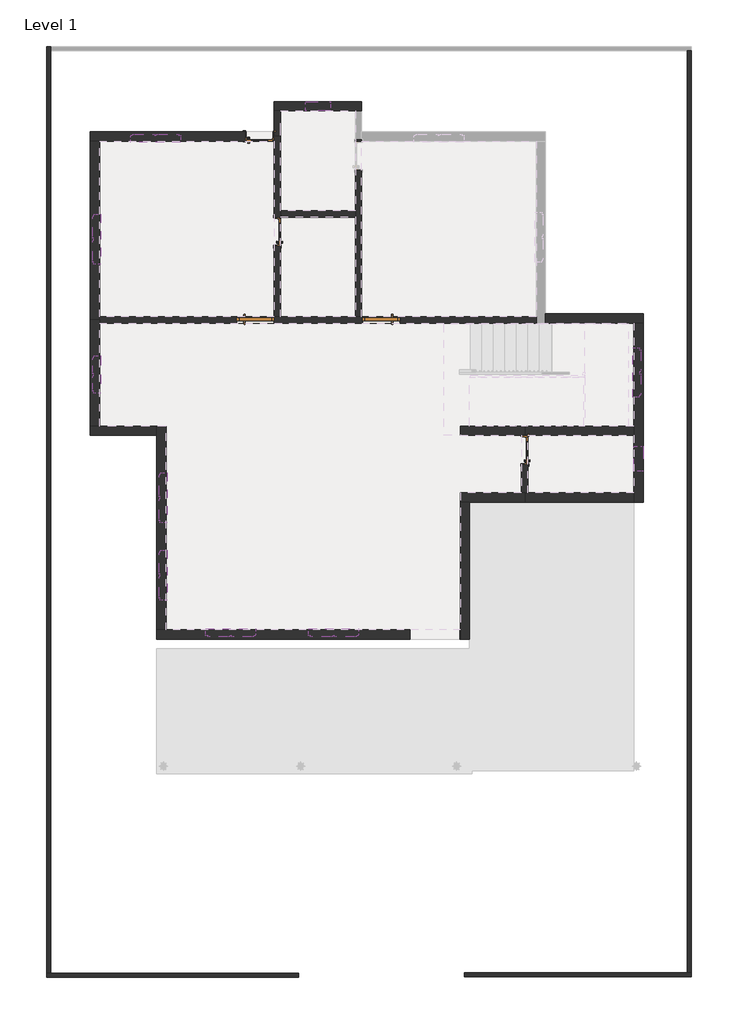
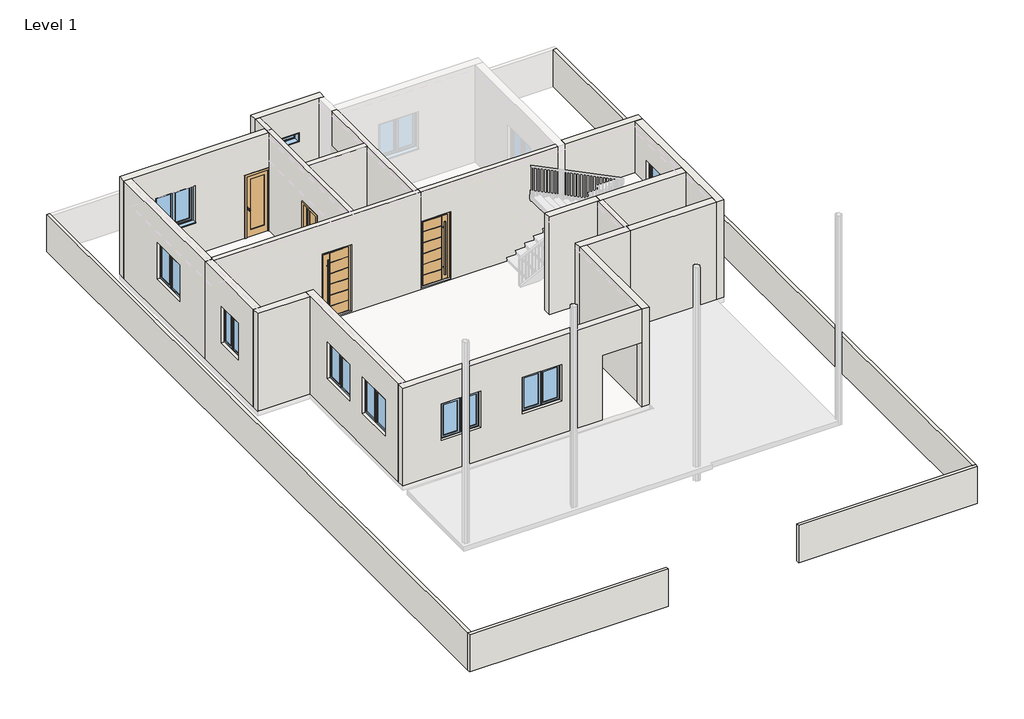
# One storey, part 1 of 2: 25 walls, 10 windows, 5 doors.
"""IFC4 building model written with IfcOpenShell, lengths in millimetres."""

from ifc_helpers import new_model, si_unit, frame, origin, origin_with_axes, place, context, project, spatial, polyline, outline, extrude, faceted_brep, transform, mapped, element, save
from components import door_3_5c4206ef, door_3_79df91aa, door_acb0f330, door_a93bef0d, awning_casement_double_3_b8244aec, awning_casement_double_4_37d249be, fixed_2_8c8825d0

model = new_model("IFC4")

# Units and contexts
model_context = context("Model", 3, world=origin())
ifc_project = project(units=[si_unit("LENGTHUNIT", "METRE", prefix="MILLI")], contexts=[model_context])

# Site, building, storey
site = spatial("IfcSite", under=ifc_project)
building = spatial("IfcBuilding", under=site)
storey = spatial("IfcBuildingStorey", under=building, Name="Level 1", Elevation=0.0)

# Doors
placement = place(None, origin())
door_3_shape = door_3_5c4206ef(model_context)
element("IfcDoor", 1, ObjectType="3'", at=placement, inside=storey, context=model_context, shape_type="MappedRepresentation", body=[
    mapped(door_3_shape, transform((-17915.4535712, 3438.0393562, 198.6445349), x_axis=(1.0, 0.0, 0.0), y_axis=(0.0, 1.0, 0.0), z_axis=(0.0, 0.0, 1.0))),
])
door_3_2_shape = door_3_79df91aa(model_context)
element("IfcDoor", 2, ObjectType="3'", at=placement, inside=storey, context=model_context, shape_type="MappedRepresentation", body=[
    mapped(door_3_2_shape, transform((-14842.0535712, 3438.0393562, 198.6445349), x_axis=(-1.0, 0.0, 0.0), y_axis=(0.0, -1.0, 0.0), z_axis=(0.0, 0.0, 1.0))),
])
door_shape = door_acb0f330(model_context)
element("IfcDoor", 3, ObjectType="M_Door-Interior-Single-1_Panel-Wood : 2'2\"", at=placement, inside=storey, context=model_context, shape_type="MappedRepresentation", body=[
    mapped(door_shape, transform((-17378.8785712, 5597.0393562, 152.4), x_axis=(0.0, 1.0, 0.0), y_axis=(-1.0, 0.0, 0.0), z_axis=(0.0, 0.0, 1.0))),
])
element("IfcDoor", 4, ObjectType="M_Door-Interior-Single-1_Panel-Wood : 2'2\"", at=placement, inside=storey, context=model_context, shape_type="MappedRepresentation", body=[
    mapped(door_shape, transform((-11333.6785712, 263.0393562, 152.4), x_axis=(0.0, 1.0, 0.0), y_axis=(-1.0, 0.0, 0.0), z_axis=(0.0, 0.0, 1.0))),
])
door_2_shape = door_a93bef0d(model_context)
element("IfcDoor", 5, ObjectType="M_Door-Interior-Single-1_Panel-Wood : 2'2\"", at=placement, inside=storey, context=model_context, shape_type="MappedRepresentation", body=[
    mapped(door_2_shape, transform((-17814.3447825, 7917.9643562, 152.4), x_axis=(1.0, 0.0, 0.0), y_axis=(0.0, 1.0, 0.0), z_axis=(0.0, 0.0, 1.0))),
])

# Walls
element("IfcWall", 6, ObjectType="Generic - 4\"", at=placement, inside=storey, context=model_context, shape_type="Brep", body=[
    faceted_brep([(-22914.3713098, -12513.1606438, 0.0), (-22914.3713098, 10013.1503619, 0.0), (-22914.3713098, 10114.7503619, 0.0), (-22914.3713098, 10114.7503619, 1219.2), (-22914.3713098, 10013.1503619, 1219.2), (-22914.3713098, -12513.1606438, 1219.2), (-23015.9713098, -12513.1606438, 0.0), (-23015.9713098, -12513.1606438, 1219.2), (-23015.9713098, 10114.7503619, 1219.2), (-23015.9713098, 10114.7503619, 0.0)], [[[0, 1, 2, 3, 4, 5]], [[6, 7, 8, 9]], [[2, 1, 0, 6, 9]], [[5, 4, 3, 8, 7]], [[3, 2, 9, 8]], [[0, 5, 7, 6]]]),
])
element("IfcWall", 7, ObjectType="Generic - 4\"", at=placement, inside=storey, context=model_context, shape_type="SweptSolid", body=[
    extrude(outline(polyline([(-7369.5713098, -12500.4606438), (-7369.5713098, 10013.1503619), (-7267.9713098, 10013.1503619), (-7267.9713098, -12500.4606438), (-7369.5713098, -12500.4606438)])), origin_with_axes(), (0.0, 0.0, 1.0), 1219.2),
])
element("IfcWall", 8, ObjectType="Generic - 4\"", at=placement, inside=storey, context=model_context, shape_type="Brep", body=[
    faceted_brep([(-12810.0535712, -12602.0606438, 0.0), (-7267.9713098, -12602.0606438, 0.0), (-7267.9713098, -12602.0606438, 1219.2), (-12810.0535712, -12602.0606438, 1219.2), (-12810.0535712, -12500.4606438, 0.0), (-12810.0535712, -12500.4606438, 1219.2), (-7369.5713098, -12500.4606438, 1219.2), (-7267.9713098, -12500.4606438, 1219.2), (-7267.9713098, -12500.4606438, 0.0), (-7369.5713098, -12500.4606438, 0.0)], [[[0, 1, 2, 3]], [[4, 5, 6, 7, 8, 9]], [[1, 0, 4, 9, 8]], [[3, 2, 7, 6, 5]], [[0, 3, 5, 4]], [[2, 1, 8, 7]]]),
])
element("IfcWall", 9, ObjectType="Generic - 4\"", at=placement, inside=storey, context=model_context, shape_type="Brep", body=[
    faceted_brep([(-23020.8535712, -12614.7606438, 0.0), (-16862.6354523, -12614.7606438, 0.0), (-16862.6354523, -12614.7606438, 1219.2), (-23020.8535712, -12614.7606438, 1219.2), (-23020.8535712, -12513.1606438, 0.0), (-23020.8535712, -12513.1606438, 1219.2), (-23015.9713098, -12513.1606438, 1219.2), (-22914.3713098, -12513.1606438, 1219.2), (-16862.6354523, -12513.1606438, 1219.2), (-16862.6354523, -12513.1606438, 0.0), (-22914.3713098, -12513.1606438, 0.0), (-23015.9713098, -12513.1606438, 0.0)], [[[0, 1, 2, 3]], [[4, 5, 6, 7, 8, 9, 10, 11]], [[1, 0, 4, 11, 10, 9]], [[2, 1, 9, 8]], [[3, 2, 8, 7, 6, 5]], [[0, 3, 5, 4]]]),
])
element("IfcWall", 10, ObjectType="Generic - 6\"", at=placement, inside=storey, context=model_context, shape_type="Brep", body=[
    faceted_brep([(-11057.4535712, 3514.2393562, 152.4), (-15311.9535712, 3514.2393562, 152.4), (-15311.9535712, 3514.2393562, 3352.8), (-11057.4535712, 3514.2393562, 3352.8), (-14384.8535712, 3514.2393562, 2388.1445349), (-15299.2535712, 3514.2393562, 2388.1445349), (-15299.2535712, 3514.2393562, 198.6445349), (-14384.8535712, 3514.2393562, 198.6445349), (-15311.9535712, 3361.8393562, 152.4), (-11057.4535712, 3361.8393562, 152.4), (-11057.4535712, 3361.8393562, 3352.8), (-15311.9535712, 3361.8393562, 3352.8), (-15299.2535712, 3361.8393562, 2388.1445349), (-14384.8535712, 3361.8393562, 2388.1445349), (-14384.8535712, 3361.8393562, 198.6445349), (-15299.2535712, 3361.8393562, 198.6445349), (-15311.9535712, 3417.2393562, 198.6445349), (-15311.9535712, 3494.2393562, 198.6445349), (-15311.9535712, 3494.2393562, 2403.1445349), (-15311.9535712, 3417.2393562, 2403.1445349), (-14384.8535712, 3494.2393562, 2388.1445349), (-15299.2535712, 3494.2393562, 2388.1445349), (-15299.2535712, 3417.2393562, 2388.1445349), (-14384.8535712, 3417.2393562, 2388.1445349), (-15299.2535712, 3494.2393562, 198.6445349), (-15299.2535712, 3417.2393562, 198.6445349), (-14384.8535712, 3417.2393562, 198.6445349), (-14369.8535712, 3417.2393562, 198.6445349), (-14369.8535712, 3494.2393562, 198.6445349), (-14384.8535712, 3494.2393562, 198.6445349), (-14369.8535712, 3494.2393562, 2403.1445349), (-14369.8535712, 3417.2393562, 2403.1445349)], [[[0, 1, 2, 3], [4, 5, 6, 7]], [[8, 9, 10, 11], [12, 13, 14, 15]], [[1, 0, 9, 8]], [[2, 1, 8, 11], [16, 17, 18, 19]], [[3, 2, 11, 10]], [[0, 3, 10, 9]], [[4, 20, 21, 5]], [[12, 22, 23, 13]], [[5, 21, 24, 6]], [[22, 12, 15, 25]], [[6, 24, 17, 16, 25, 15, 14, 26, 27, 28, 29, 7]], [[20, 4, 7, 29]], [[13, 23, 26, 14]], [[30, 31, 19, 18]], [[23, 22, 25, 16, 19, 31, 27, 26]], [[28, 27, 31, 30]], [[21, 20, 29, 28, 30, 18, 17, 24]]]),
])
element("IfcWall", 11, ObjectType="Generic - 6\"", at=placement, inside=storey, context=model_context, shape_type="Brep", body=[
    faceted_brep([(-17305.8535712, 7921.1393562, 152.4), (-17305.8535712, 7921.1393562, 3352.8), (-17305.8535712, 6105.0393562, 3352.8), (-17305.8535712, 5952.6393562, 3352.8), (-17305.8535712, 3514.2393562, 3352.8), (-17305.8535712, 3514.2393562, 152.4), (-17305.8535712, 5241.8393562, 152.4), (-17305.8535712, 5241.8393562, 2177.4), (-17305.8535712, 5952.2393562, 2177.4), (-17305.8535712, 5952.2393562, 152.4), (-17305.8535712, 5952.6393562, 152.4), (-17305.8535712, 6105.0393562, 152.4), (-17458.2535712, 7921.1393562, 3352.8), (-17458.2535712, 7921.1393562, 152.4), (-17458.2535712, 7806.8393562, 152.4), (-17458.2535712, 5952.2393562, 152.4), (-17458.2535712, 5952.2393562, 2177.4), (-17458.2535712, 5241.8393562, 2177.4), (-17458.2535712, 5241.8393562, 152.4), (-17458.2535712, 3514.2393562, 152.4), (-17458.2535712, 3514.2393562, 198.6445349), (-17458.2535712, 3514.2393562, 2388.1445349), (-17458.2535712, 3514.2393562, 3352.8), (-17458.2535712, 7806.8393562, 3352.8)], [[[0, 1, 2, 3, 4, 5, 6, 7, 8, 9, 10, 11]], [[12, 13, 14, 15, 16, 17, 18, 19, 20, 21, 22, 23]], [[5, 19, 18, 6]], [[13, 0, 11, 10, 9, 15, 14]], [[1, 0, 13, 12]], [[4, 3, 2, 1, 12, 23, 22]], [[5, 4, 22, 21, 20, 19]], [[8, 16, 15, 9]], [[16, 8, 7, 17]], [[17, 7, 6, 18]]]),
])
element("IfcWall", 12, ObjectType="Generic - 6\"", at=placement, inside=storey, context=model_context, shape_type="SweptSolid", body=[
    extrude(outline(polyline([(-15477.0535712, 5952.6393562), (-17305.8535712, 5952.6393562), (-17305.8535712, 6105.0393562), (-15477.0535712, 6105.0393562), (-15477.0535712, 5952.6393562)])), frame((0.0, 0.0, 152.4), z_axis=(0.0, 0.0, 1.0), x_axis=(1.0, 0.0, 0.0)), (0.0, 0.0, 1.0), 3200.4),
])
element("IfcWall", 13, ObjectType="Generic - 6\"", at=placement, inside=storey, context=model_context, shape_type="Brep", body=[
    faceted_brep([(-11260.6535712, 618.6393562, 3352.8), (-11260.6535712, -778.3606438, 3352.8), (-11260.6535712, -778.3606438, 152.4), (-11260.6535712, -92.1606438, 152.4), (-11260.6535712, -92.1606438, 2177.4), (-11260.6535712, 618.2393562, 2177.4), (-11260.6535712, 618.2393562, 152.4), (-11260.6535712, 618.6393562, 152.4), (-11413.0535712, -778.3606438, 3352.8), (-11413.0535712, 618.6393562, 3352.8), (-11413.0535712, 618.6393562, 152.4), (-11413.0535712, 618.2393562, 152.4), (-11413.0535712, 618.2393562, 2177.4), (-11413.0535712, -92.1606438, 2177.4), (-11413.0535712, -92.1606438, 152.4), (-11413.0535712, -778.3606438, 152.4), (-11336.8535712, 618.6393562, 152.4), (-11336.8535712, -778.3606438, 152.4), (-11336.8535712, 618.6393562, 3352.8), (-11336.8535712, -778.3606438, 3352.8)], [[[0, 1, 2, 3, 4, 5, 6, 7]], [[8, 9, 10, 11, 12, 13, 14, 15]], [[10, 16, 7, 6, 11]], [[2, 17, 15, 14, 3]], [[1, 0, 18, 9, 8, 19]], [[2, 1, 19, 8, 15, 17]], [[0, 7, 16, 10, 9, 18]], [[5, 12, 11, 6]], [[12, 5, 4, 13]], [[13, 4, 3, 14]]]),
])
element("IfcWall", 14, ObjectType="Generic - 6\"", at=placement, inside=storey, context=model_context, shape_type="Brep", body=[
    faceted_brep([(-15311.9535712, 3514.2393562, 152.4), (-15324.6535712, 3514.2393562, 152.4), (-15477.0535712, 3514.2393562, 152.4), (-17305.8535712, 3514.2393562, 152.4), (-17458.2535712, 3514.2393562, 152.4), (-21725.4535712, 3514.2393562, 152.4), (-21725.4535712, 3514.2393562, 3352.8), (-17458.2535712, 3514.2393562, 3352.8), (-17305.8535712, 3514.2393562, 3352.8), (-15477.0535712, 3514.2393562, 3352.8), (-15324.6535712, 3514.2393562, 3352.8), (-15311.9535712, 3514.2393562, 3352.8), (-17458.2535712, 3514.2393562, 2388.1445349), (-18372.6535712, 3514.2393562, 2388.1445349), (-18372.6535712, 3514.2393562, 198.6445349), (-17458.2535712, 3514.2393562, 198.6445349), (-21725.4535712, 3361.8393562, 152.4), (-15311.9535712, 3361.8393562, 152.4), (-15311.9535712, 3361.8393562, 3352.8), (-21725.4535712, 3361.8393562, 3352.8), (-18372.6535712, 3361.8393562, 2388.1445349), (-17458.2535712, 3361.8393562, 2388.1445349), (-17458.2535712, 3361.8393562, 198.6445349), (-18372.6535712, 3361.8393562, 198.6445349), (-21725.4535712, 3438.0393562, 152.4), (-21725.4535712, 3438.0393562, 3352.8), (-15311.9535712, 3494.2393562, 198.6445349), (-15311.9535712, 3417.2393562, 198.6445349), (-15311.9535712, 3417.2393562, 2403.1445349), (-15311.9535712, 3494.2393562, 2403.1445349), (-18372.6535712, 3417.2393562, 2388.1445349), (-17458.2535712, 3417.2393562, 2388.1445349), (-18372.6535712, 3494.2393562, 2388.1445349), (-17458.2535712, 3494.2393562, 2388.1445349), (-17458.2535712, 3417.2393562, 198.6445349), (-17458.2535712, 3494.2393562, 198.6445349), (-18372.6535712, 3494.2393562, 198.6445349), (-18387.6535712, 3494.2393562, 198.6445349), (-18387.6535712, 3417.2393562, 198.6445349), (-18372.6535712, 3417.2393562, 198.6445349), (-17443.2535712, 3417.2393562, 198.6445349), (-17443.2535712, 3494.2393562, 198.6445349), (-18387.6535712, 3494.2393562, 2403.1445349), (-17443.2535712, 3494.2393562, 2403.1445349), (-17443.2535712, 3417.2393562, 2403.1445349), (-18387.6535712, 3417.2393562, 2403.1445349), (-15314.2535712, 3494.2393562, 198.6445349), (-15314.2535712, 3417.2393562, 198.6445349), (-15314.2535712, 3417.2393562, 2403.1445349), (-15314.2535712, 3494.2393562, 2403.1445349)], [[[0, 1, 2, 3, 4, 5, 6, 7, 8, 9, 10, 11], [12, 13, 14, 15]], [[16, 17, 18, 19], [20, 21, 22, 23]], [[5, 4, 3, 2, 1, 0, 17, 16, 24]], [[11, 10, 9, 8, 7, 6, 25, 19, 18]], [[0, 11, 18, 17], [26, 27, 28, 29]], [[6, 5, 24, 16, 19, 25]], [[20, 30, 31, 21]], [[32, 13, 12, 33]], [[21, 31, 34, 22]], [[33, 12, 15, 35]], [[36, 37, 38, 39, 23, 22, 34, 40, 41, 35, 15, 14]], [[30, 20, 23, 39]], [[13, 32, 36, 14]], [[42, 43, 44, 45]], [[44, 43, 41, 40]], [[39, 38, 45, 44, 40, 34, 31, 30]], [[38, 37, 42, 45]], [[37, 36, 32, 33, 35, 41, 43, 42]], [[46, 47, 27, 26]], [[48, 49, 29, 28]], [[47, 46, 49, 48]], [[47, 48, 28, 27]], [[49, 46, 26, 29]]]),
])
element("IfcWall", 15, ObjectType="Generic - 6\"", at=placement, inside=storey, context=model_context, shape_type="Brep", body=[
    faceted_brep([(-15477.0535712, 3514.2393562, 3352.8), (-15477.0535712, 5952.6393562, 3352.8), (-15477.0535712, 6105.0393562, 3352.8), (-15477.0535712, 7844.9393562, 3352.8), (-15477.0535712, 7844.9393562, 152.4), (-15477.0535712, 7800.0893562, 152.4), (-15477.0535712, 7800.0893562, 2177.4), (-15477.0535712, 7089.6893562, 2177.4), (-15477.0535712, 7089.6893562, 152.4), (-15477.0535712, 6105.0393562, 152.4), (-15477.0535712, 5952.6393562, 152.4), (-15477.0535712, 3514.2393562, 152.4), (-15324.6535712, 7844.9393562, 3352.8), (-15324.6535712, 3514.2393562, 3352.8), (-15324.6535712, 3514.2393562, 152.4), (-15324.6535712, 7089.6893562, 152.4), (-15324.6535712, 7089.6893562, 2177.4), (-15324.6535712, 7800.0893562, 2177.4), (-15324.6535712, 7800.0893562, 152.4), (-15324.6535712, 7844.9393562, 152.4)], [[[0, 1, 2, 3, 4, 5, 6, 7, 8, 9, 10, 11]], [[12, 13, 14, 15, 16, 17, 18, 19]], [[14, 11, 10, 9, 8, 15]], [[4, 19, 18, 5]], [[3, 2, 1, 0, 13, 12]], [[4, 3, 12, 19]], [[0, 11, 14, 13]], [[17, 6, 5, 18]], [[6, 17, 16, 7]], [[7, 16, 15, 8]]]),
])
element("IfcWall", 16, ObjectType="Generic - 6\"", at=placement, inside=storey, context=model_context, shape_type="Brep", body=[
    faceted_brep([(-17305.8535712, 7921.1393562, 152.4), (-17305.8535712, 8543.4393562, 152.4), (-17305.8535712, 8543.4393562, 3352.8), (-17305.8535712, 7921.1393562, 3352.8), (-17458.2535712, 7921.1393562, 152.4), (-17458.2535712, 7921.1393562, 3352.8), (-17458.2535712, 8035.4393562, 3352.8), (-17458.2535712, 8543.4393562, 3352.8), (-17458.2535712, 8543.4393562, 152.4), (-17458.2535712, 8035.4393562, 152.4)], [[[0, 1, 2, 3]], [[4, 5, 6, 7, 8, 9]], [[1, 0, 4, 9, 8]], [[3, 2, 7, 6, 5]], [[0, 3, 5, 4]], [[2, 1, 8, 7]]]),
])
element("IfcWall", 17, ObjectType="Generic - 9\"", at=placement, inside=storey, context=model_context, shape_type="Brep", body=[
    faceted_brep([(-17458.2535712, 7806.8393562, 3352.8), (-21725.4535712, 7806.8393562, 3352.8), (-21954.0535712, 7806.8393562, 3352.8), (-21954.0535712, 7806.8393562, 152.4), (-21725.4535712, 7806.8393562, 152.4), (-18169.5447825, 7806.8393562, 152.4), (-18169.5447825, 7806.8393562, 2177.4), (-17459.1447825, 7806.8393562, 2177.4), (-17459.1447825, 7806.8393562, 152.4), (-17458.2535712, 7806.8393562, 152.4), (-19744.2535712, 7806.8393562, 1219.2), (-20963.4535712, 7806.8393562, 1219.2), (-20963.4535712, 7806.8393562, 2419.2), (-19744.2535712, 7806.8393562, 2419.2), (-21954.0535712, 8035.4393562, 3352.8), (-17458.2535712, 8035.4393562, 3352.8), (-17458.2535712, 8035.4393562, 152.4), (-17459.1447825, 8035.4393562, 152.4), (-17459.1447825, 8035.4393562, 2177.4), (-18169.5447825, 8035.4393562, 2177.4), (-18169.5447825, 8035.4393562, 152.4), (-21954.0535712, 8035.4393562, 152.4), (-19744.2535712, 8035.4393562, 1219.2), (-19744.2535712, 8035.4393562, 2419.2), (-20963.4535712, 8035.4393562, 2419.2), (-20963.4535712, 8035.4393562, 1219.2), (-17458.2535712, 7921.1393562, 152.4), (-17458.2535712, 7921.1393562, 3352.8)], [[[0, 1, 2, 3, 4, 5, 6, 7, 8, 9], [10, 11, 12, 13]], [[14, 15, 16, 17, 18, 19, 20, 21], [22, 23, 24, 25]], [[3, 21, 20, 5, 4]], [[16, 26, 9, 8, 17]], [[2, 1, 0, 27, 15, 14]], [[3, 2, 14, 21]], [[23, 22, 10, 13]], [[24, 23, 13, 12]], [[25, 24, 12, 11]], [[22, 25, 11, 10]], [[7, 18, 17, 8]], [[18, 7, 6, 19]], [[19, 6, 5, 20]], [[0, 9, 26, 16, 15, 27]]]),
])
element("IfcWall", 18, ObjectType="Generic - 9\"", at=placement, inside=storey, context=model_context, shape_type="Brep", body=[
    faceted_brep([(-17458.2535712, 8543.4393562, 152.4), (-17305.8535712, 8543.4393562, 152.4), (-15477.0535712, 8543.4393562, 152.4), (-15324.6535712, 8543.4393562, 152.4), (-15324.6535712, 8543.4393562, 3352.8), (-15477.0535712, 8543.4393562, 3352.8), (-17305.8535712, 8543.4393562, 3352.8), (-17458.2535712, 8543.4393562, 3352.8), (-16086.6535712, 8543.4393562, 2438.4), (-16086.6535712, 8543.4393562, 2133.6), (-16696.2535712, 8543.4393562, 2133.6), (-16696.2535712, 8543.4393562, 2438.4), (-17458.2535712, 8772.0393562, 152.4), (-17458.2535712, 8772.0393562, 3352.8), (-15324.6535712, 8772.0393562, 3352.8), (-15324.6535712, 8772.0393562, 152.4), (-16086.6535712, 8772.0393562, 2438.4), (-16696.2535712, 8772.0393562, 2438.4), (-16696.2535712, 8772.0393562, 2133.6), (-16086.6535712, 8772.0393562, 2133.6)], [[[0, 1, 2, 3, 4, 5, 6, 7], [8, 9, 10, 11]], [[12, 13, 14, 15], [16, 17, 18, 19]], [[3, 2, 1, 0, 12, 15]], [[7, 6, 5, 4, 14, 13]], [[4, 3, 15, 14]], [[0, 7, 13, 12]], [[9, 8, 16, 19]], [[10, 9, 19, 18]], [[11, 10, 18, 17]], [[8, 11, 17, 16]]]),
])
element("IfcWall", 19, ObjectType="Generic - 9\"", at=placement, inside=storey, context=model_context, shape_type="Brep", body=[
    faceted_brep([(-10828.8535712, 3361.8393562, 152.4), (-8669.8535712, 3361.8393562, 152.4), (-8441.2535712, 3361.8393562, 152.4), (-8441.2535712, 3361.8393562, 3352.8), (-8669.8535712, 3361.8393562, 3352.8), (-10828.8535712, 3361.8393562, 3352.8), (-10828.8535712, 3590.4393562, 152.4), (-10828.8535712, 3590.4393562, 3352.8), (-8441.2535712, 3590.4393562, 3352.8), (-8441.2535712, 3590.4393562, 152.4)], [[[0, 1, 2, 3, 4, 5]], [[6, 7, 8, 9]], [[2, 1, 0, 6, 9]], [[5, 4, 3, 8, 7]], [[0, 5, 7, 6]], [[3, 2, 9, 8]]]),
])
element("IfcWall", 20, ObjectType="Generic - 9\"", at=placement, inside=storey, context=model_context, shape_type="Brep", body=[
    faceted_brep([(-8669.8535712, 3361.8393562, 152.4), (-8669.8535712, 847.2393562, 152.4), (-8669.8535712, 618.6393562, 152.4), (-8669.8535712, -778.3606438, 152.4), (-8669.8535712, -1006.9606438, 152.4), (-8669.8535712, -1006.9606438, 3352.8), (-8669.8535712, -778.3606438, 3352.8), (-8669.8535712, 618.6393562, 3352.8), (-8669.8535712, 847.2393562, 3352.8), (-8669.8535712, 3361.8393562, 3352.8), (-8669.8535712, 1545.7393562, 1219.2), (-8669.8535712, 2764.9393562, 1219.2), (-8669.8535712, 2764.9393562, 2419.2), (-8669.8535712, 1545.7393562, 2419.2), (-8669.8535712, -257.6606438, 2438.4), (-8669.8535712, -257.6606438, 2133.6), (-8669.8535712, 351.9393562, 2133.6), (-8669.8535712, 351.9393562, 2438.4), (-8441.2535712, 3361.8393562, 152.4), (-8441.2535712, 3361.8393562, 3352.8), (-8441.2535712, -1006.9606438, 3352.8), (-8441.2535712, -1006.9606438, 152.4), (-8441.2535712, 1545.7393562, 1219.2), (-8441.2535712, 1545.7393562, 2419.2), (-8441.2535712, 2764.9393562, 2419.2), (-8441.2535712, 2764.9393562, 1219.2), (-8441.2535712, -257.6606438, 2438.4), (-8441.2535712, 351.9393562, 2438.4), (-8441.2535712, 351.9393562, 2133.6), (-8441.2535712, -257.6606438, 2133.6)], [[[0, 1, 2, 3, 4, 5, 6, 7, 8, 9], [10, 11, 12, 13], [14, 15, 16, 17]], [[18, 19, 20, 21], [22, 23, 24, 25], [26, 27, 28, 29]], [[4, 3, 2, 1, 0, 18, 21]], [[9, 8, 7, 6, 5, 20, 19]], [[0, 9, 19, 18]], [[5, 4, 21, 20]], [[23, 22, 10, 13]], [[24, 23, 13, 12]], [[25, 24, 12, 11]], [[22, 25, 11, 10]], [[15, 14, 26, 29]], [[16, 15, 29, 28]], [[17, 16, 28, 27]], [[14, 17, 27, 26]]]),
])
element("IfcWall", 21, ObjectType="Generic - 9\"", at=placement, inside=storey, context=model_context, shape_type="Brep", body=[
    faceted_brep([(-8669.8535712, -778.3606438, 152.4), (-11260.6535712, -778.3606438, 152.4), (-11336.8535712, -778.3606438, 152.4), (-11336.8535712, -778.3606438, 3352.8), (-11260.6535712, -778.3606438, 3352.8), (-8669.8535712, -778.3606438, 3352.8), (-8669.8535712, -1006.9606438, 152.4), (-8669.8535712, -1006.9606438, 3352.8), (-11336.8535712, -1006.9606438, 3352.8), (-11336.8535712, -1006.9606438, 152.4)], [[[0, 1, 2, 3, 4, 5]], [[6, 7, 8, 9]], [[2, 1, 0, 6, 9]], [[3, 2, 9, 8]], [[5, 4, 3, 8, 7]], [[0, 5, 7, 6]]]),
])
element("IfcWall", 22, ObjectType="Generic - 9\"", at=placement, inside=storey, context=model_context, shape_type="Brep", body=[
    faceted_brep([(-12911.6535712, -1006.9606438, 152.4), (-12911.6535712, -4131.1606438, 152.4), (-12911.6535712, -4359.7606438, 152.4), (-12911.6535712, -4359.7606438, 3352.8), (-12911.6535712, -4131.1606438, 3352.8), (-12911.6535712, -1006.9606438, 3352.8), (-12683.0535712, -1006.9606438, 152.4), (-12683.0535712, -1006.9606438, 3352.8), (-12683.0535712, -4359.7606438, 3352.8), (-12683.0535712, -4359.7606438, 152.4)], [[[0, 1, 2, 3, 4, 5]], [[6, 7, 8, 9]], [[2, 1, 0, 6, 9]], [[5, 4, 3, 8, 7]], [[0, 5, 7, 6]], [[3, 2, 9, 8]]]),
])
element("IfcWall", 23, ObjectType="Generic - 9\"", at=placement, inside=storey, context=model_context, shape_type="Brep", body=[
    faceted_brep([(-12911.6535712, -4359.7606438, 3352.8), (-20328.4535712, -4359.7606438, 3352.8), (-20328.4535712, -4359.7606438, 152.4), (-14143.5535712, -4359.7606438, 152.4), (-14143.5535712, -4359.7606438, 2262.4), (-12924.3535712, -4359.7606438, 2262.4), (-12924.3535712, -4359.7606438, 152.4), (-12911.6535712, -4359.7606438, 152.4), (-19128.3035712, -4359.7606438, 1219.2), (-19128.3035712, -4359.7606438, 2419.2), (-17909.1035712, -4359.7606438, 2419.2), (-17909.1035712, -4359.7606438, 1219.2), (-16620.0535712, -4359.7606438, 1219.2), (-16620.0535712, -4359.7606438, 2419.2), (-15400.8535712, -4359.7606438, 2419.2), (-15400.8535712, -4359.7606438, 1219.2), (-20328.4535712, -4131.1606438, 3352.8), (-20099.8535712, -4131.1606438, 3352.8), (-12911.6535712, -4131.1606438, 3352.8), (-12911.6535712, -4131.1606438, 152.4), (-12924.3535712, -4131.1606438, 152.4), (-12924.3535712, -4131.1606438, 2262.4), (-14143.5535712, -4131.1606438, 2262.4), (-14143.5535712, -4131.1606438, 152.4), (-20099.8535712, -4131.1606438, 152.4), (-20328.4535712, -4131.1606438, 152.4), (-19128.3035712, -4131.1606438, 1219.2), (-17909.1035712, -4131.1606438, 1219.2), (-17909.1035712, -4131.1606438, 2419.2), (-19128.3035712, -4131.1606438, 2419.2), (-16620.0535712, -4131.1606438, 1219.2), (-15400.8535712, -4131.1606438, 1219.2), (-15400.8535712, -4131.1606438, 2419.2), (-16620.0535712, -4131.1606438, 2419.2)], [[[0, 1, 2, 3, 4, 5, 6, 7], [8, 9, 10, 11], [12, 13, 14, 15]], [[16, 17, 18, 19, 20, 21, 22, 23, 24, 25], [26, 27, 28, 29], [30, 31, 32, 33]], [[19, 7, 6, 20]], [[2, 25, 24, 23, 3]], [[1, 0, 18, 17, 16]], [[0, 7, 19, 18]], [[2, 1, 16, 25]], [[9, 8, 26, 29]], [[10, 9, 29, 28]], [[11, 10, 28, 27]], [[8, 11, 27, 26]], [[13, 12, 30, 33]], [[14, 13, 33, 32]], [[15, 14, 32, 31]], [[12, 15, 31, 30]], [[5, 21, 20, 6]], [[22, 4, 3, 23]], [[21, 5, 4, 22]]]),
])
element("IfcWall", 24, ObjectType="Generic - 9\"", at=placement, inside=storey, context=model_context, shape_type="Brep", body=[
    faceted_brep([(-20099.8535712, -4131.1606438, 152.4), (-20099.8535712, 847.2393562, 152.4), (-20099.8535712, 847.2393562, 3352.8), (-20099.8535712, -4131.1606438, 3352.8), (-20099.8535712, -295.7606438, 1219.2), (-20099.8535712, -1514.9606438, 1219.2), (-20099.8535712, -1514.9606438, 2419.2), (-20099.8535712, -295.7606438, 2419.2), (-20099.8535712, -2188.0606438, 1219.2), (-20099.8535712, -3407.2606438, 1219.2), (-20099.8535712, -3407.2606438, 2419.2), (-20099.8535712, -2188.0606438, 2419.2), (-20328.4535712, -4131.1606438, 152.4), (-20328.4535712, -4131.1606438, 3352.8), (-20328.4535712, 618.6393562, 3352.8), (-20328.4535712, 847.2393562, 3352.8), (-20328.4535712, 847.2393562, 152.4), (-20328.4535712, 618.6393562, 152.4), (-20328.4535712, -295.7606438, 1219.2), (-20328.4535712, -295.7606438, 2419.2), (-20328.4535712, -1514.9606438, 2419.2), (-20328.4535712, -1514.9606438, 1219.2), (-20328.4535712, -2188.0606438, 1219.2), (-20328.4535712, -2188.0606438, 2419.2), (-20328.4535712, -3407.2606438, 2419.2), (-20328.4535712, -3407.2606438, 1219.2)], [[[0, 1, 2, 3], [4, 5, 6, 7], [8, 9, 10, 11]], [[12, 13, 14, 15, 16, 17], [18, 19, 20, 21], [22, 23, 24, 25]], [[1, 0, 12, 17, 16]], [[3, 2, 15, 14, 13]], [[0, 3, 13, 12]], [[2, 1, 16, 15]], [[19, 18, 4, 7]], [[20, 19, 7, 6]], [[21, 20, 6, 5]], [[18, 21, 5, 4]], [[23, 22, 8, 11]], [[24, 23, 11, 10]], [[25, 24, 10, 9]], [[22, 25, 9, 8]]]),
])
element("IfcWall", 25, ObjectType="Generic - 9\"", at=placement, inside=storey, context=model_context, shape_type="Brep", body=[
    faceted_brep([(-20328.4535712, 847.2393562, 152.4), (-21725.4535712, 847.2393562, 152.4), (-21954.0535712, 847.2393562, 152.4), (-21954.0535712, 847.2393562, 3352.8), (-21725.4535712, 847.2393562, 3352.8), (-20328.4535712, 847.2393562, 3352.8), (-20328.4535712, 618.6393562, 152.4), (-20328.4535712, 618.6393562, 3352.8), (-21954.0535712, 618.6393562, 3352.8), (-21954.0535712, 618.6393562, 152.4)], [[[0, 1, 2, 3, 4, 5]], [[6, 7, 8, 9]], [[2, 1, 0, 6, 9]], [[5, 4, 3, 8, 7]], [[0, 5, 7, 6]], [[3, 2, 9, 8]]]),
])
element("IfcWall", 26, ObjectType="Generic - 9\"", at=placement, inside=storey, context=model_context, shape_type="Brep", body=[
    faceted_brep([(-21725.4535712, 847.2393562, 152.4), (-21725.4535712, 3361.8393562, 152.4), (-21725.4535712, 3438.0393562, 152.4), (-21725.4535712, 3438.0393562, 3352.8), (-21725.4535712, 3361.8393562, 3352.8), (-21725.4535712, 847.2393562, 3352.8), (-21725.4535712, 2561.7393562, 1219.2), (-21725.4535712, 1647.3393562, 1219.2), (-21725.4535712, 1647.3393562, 2419.2), (-21725.4535712, 2561.7393562, 2419.2), (-21954.0535712, 847.2393562, 152.4), (-21954.0535712, 847.2393562, 3352.8), (-21954.0535712, 3438.0393562, 3352.8), (-21954.0535712, 3438.0393562, 152.4), (-21954.0535712, 2561.7393562, 1219.2), (-21954.0535712, 2561.7393562, 2419.2), (-21954.0535712, 1647.3393562, 2419.2), (-21954.0535712, 1647.3393562, 1219.2)], [[[0, 1, 2, 3, 4, 5], [6, 7, 8, 9]], [[10, 11, 12, 13], [14, 15, 16, 17]], [[2, 1, 0, 10, 13]], [[3, 2, 13, 12]], [[5, 4, 3, 12, 11]], [[0, 5, 11, 10]], [[15, 14, 6, 9]], [[16, 15, 9, 8]], [[17, 16, 8, 7]], [[14, 17, 7, 6]]]),
])
element("IfcWall", 27, ObjectType="Generic - 9\"", at=placement, inside=storey, context=model_context, shape_type="Brep", body=[
    faceted_brep([(-12911.6535712, 618.6393562, 152.4), (-11413.0535712, 618.6393562, 152.4), (-11336.8535712, 618.6393562, 152.4), (-11336.8535712, 618.6393562, 3352.8), (-11413.0535712, 618.6393562, 3352.8), (-12911.6535712, 618.6393562, 3352.8), (-12911.6535712, 847.2393562, 152.4), (-12911.6535712, 847.2393562, 3352.8), (-11336.8535712, 847.2393562, 3352.8), (-11336.8535712, 847.2393562, 152.4)], [[[0, 1, 2, 3, 4, 5]], [[6, 7, 8, 9]], [[2, 1, 0, 6, 9]], [[3, 2, 9, 8]], [[5, 4, 3, 8, 7]], [[0, 5, 7, 6]]]),
])
element("IfcWall", 28, ObjectType="Generic - 9\"", at=placement, inside=storey, context=model_context, shape_type="Brep", body=[
    faceted_brep([(-21725.4535712, 3438.0393562, 152.4), (-21725.4535712, 3514.2393562, 152.4), (-21725.4535712, 7806.8393562, 152.4), (-21725.4535712, 7806.8393562, 3352.8), (-21725.4535712, 3514.2393562, 3352.8), (-21725.4535712, 3438.0393562, 3352.8), (-21725.4535712, 6016.1393562, 1219.2), (-21725.4535712, 4796.9393562, 1219.2), (-21725.4535712, 4796.9393562, 2419.2), (-21725.4535712, 6016.1393562, 2419.2), (-21954.0535712, 3438.0393562, 152.4), (-21954.0535712, 3438.0393562, 3352.8), (-21954.0535712, 7806.8393562, 3352.8), (-21954.0535712, 7806.8393562, 152.4), (-21954.0535712, 6016.1393562, 1219.2), (-21954.0535712, 6016.1393562, 2419.2), (-21954.0535712, 4796.9393562, 2419.2), (-21954.0535712, 4796.9393562, 1219.2)], [[[0, 1, 2, 3, 4, 5], [6, 7, 8, 9]], [[10, 11, 12, 13], [14, 15, 16, 17]], [[2, 1, 0, 10, 13]], [[5, 4, 3, 12, 11]], [[0, 5, 11, 10]], [[3, 2, 13, 12]], [[14, 17, 7, 6]], [[17, 16, 8, 7]], [[16, 15, 9, 8]], [[15, 14, 6, 9]]]),
])
element("IfcWall", 29, ObjectType="Generic - 9\"", at=placement, inside=storey, context=model_context, shape_type="Brep", body=[
    faceted_brep([(-11336.8535712, 618.6393562, 152.4), (-11260.6535712, 618.6393562, 152.4), (-8669.8535712, 618.6393562, 152.4), (-8669.8535712, 618.6393562, 3352.8), (-11260.6535712, 618.6393562, 3352.8), (-11336.8535712, 618.6393562, 3352.8), (-11336.8535712, 847.2393562, 152.4), (-11336.8535712, 847.2393562, 3352.8), (-8669.8535712, 847.2393562, 3352.8), (-8669.8535712, 847.2393562, 152.4)], [[[0, 1, 2, 3, 4, 5]], [[6, 7, 8, 9]], [[2, 1, 0, 6, 9]], [[5, 4, 3, 8, 7]], [[0, 5, 7, 6]], [[3, 2, 9, 8]]]),
])
element("IfcWall", 30, ObjectType="Generic - 9\"", at=placement, inside=storey, context=model_context, shape_type="Brep", body=[
    faceted_brep([(-11336.8535712, -778.3606438, 152.4), (-11413.0535712, -778.3606438, 152.4), (-12911.6535712, -778.3606438, 152.4), (-12911.6535712, -778.3606438, 3352.8), (-11413.0535712, -778.3606438, 3352.8), (-11336.8535712, -778.3606438, 3352.8), (-11336.8535712, -1006.9606438, 152.4), (-11336.8535712, -1006.9606438, 3352.8), (-12683.0535712, -1006.9606438, 3352.8), (-12911.6535712, -1006.9606438, 3352.8), (-12911.6535712, -1006.9606438, 152.4), (-12683.0535712, -1006.9606438, 152.4)], [[[0, 1, 2, 3, 4, 5]], [[6, 7, 8, 9, 10, 11]], [[2, 1, 0, 6, 11, 10]], [[5, 4, 3, 9, 8, 7]], [[0, 5, 7, 6]], [[3, 2, 10, 9]]]),
])

# Windows
awning_casement_double_3_shape = awning_casement_double_3_b8244aec(model_context)
element("IfcWindow", 31, ObjectType="Awning Casement double : 3'", at=placement, inside=storey, context=model_context, shape_type="MappedRepresentation", body=[
    mapped(awning_casement_double_3_shape, transform((-21839.7535712, 2104.5393562, 419.2), x_axis=(0.0, -1.0, 0.0), y_axis=(1.0, 0.0, 0.0), z_axis=(0.0, 0.0, 1.0))),
])
awning_casement_double_4_shape = awning_casement_double_4_37d249be(model_context)
element("IfcWindow", 32, ObjectType="Awning Casement double : 4'", at=placement, inside=storey, context=model_context, shape_type="MappedRepresentation", body=[
    mapped(awning_casement_double_4_shape, transform((-20353.8535712, 7921.1393562, 419.2), x_axis=(-1.0, 0.0, 0.0), y_axis=(0.0, -1.0, 0.0), z_axis=(0.0, 0.0, 1.0))),
])
element("IfcWindow", 33, ObjectType="Awning Casement double : 4'", at=placement, inside=storey, context=model_context, shape_type="MappedRepresentation", body=[
    mapped(awning_casement_double_4_shape, transform((-21839.7535712, 5406.5393562, 419.2), x_axis=(0.0, -1.0, 0.0), y_axis=(1.0, 0.0, 0.0), z_axis=(0.0, 0.0, 1.0))),
])
element("IfcWindow", 34, ObjectType="Awning Casement double : 4'", at=placement, inside=storey, context=model_context, shape_type="MappedRepresentation", body=[
    mapped(awning_casement_double_4_shape, transform((-20214.1535712, -905.3606438, 419.2), x_axis=(0.0, -1.0, 0.0), y_axis=(1.0, 0.0, 0.0), z_axis=(0.0, 0.0, 1.0))),
])
element("IfcWindow", 35, ObjectType="Awning Casement double : 4'", at=placement, inside=storey, context=model_context, shape_type="MappedRepresentation", body=[
    mapped(awning_casement_double_4_shape, transform((-20214.1535712, -2797.6606438, 419.2), x_axis=(0.0, -1.0, 0.0), y_axis=(1.0, 0.0, 0.0), z_axis=(0.0, 0.0, 1.0))),
])
element("IfcWindow", 36, ObjectType="Awning Casement double : 4'", at=placement, inside=storey, context=model_context, shape_type="MappedRepresentation", body=[
    mapped(awning_casement_double_4_shape, transform((-18518.7035712, -4245.4606438, 419.2), x_axis=(1.0, 0.0, 0.0), y_axis=(0.0, 1.0, 0.0), z_axis=(0.0, 0.0, 1.0))),
])
element("IfcWindow", 37, ObjectType="Awning Casement double : 4'", at=placement, inside=storey, context=model_context, shape_type="MappedRepresentation", body=[
    mapped(awning_casement_double_4_shape, transform((-16010.4535712, -4245.4606438, 419.2), x_axis=(1.0, 0.0, 0.0), y_axis=(0.0, 1.0, 0.0), z_axis=(0.0, 0.0, 1.0))),
])
element("IfcWindow", 38, ObjectType="Awning Casement double : 4'", at=placement, inside=storey, context=model_context, shape_type="MappedRepresentation", body=[
    mapped(awning_casement_double_4_shape, transform((-8555.5535712, 2155.3393562, 419.2), x_axis=(0.0, 1.0, 0.0), y_axis=(-1.0, 0.0, 0.0), z_axis=(0.0, 0.0, 1.0))),
])
fixed_2_shape = fixed_2_8c8825d0(model_context)
element("IfcWindow", 39, ObjectType="Fixed : 2'", at=placement, inside=storey, context=model_context, shape_type="MappedRepresentation", body=[
    mapped(fixed_2_shape, transform((-8555.5535712, 9.0393562, 1219.2), x_axis=(0.0, -1.0, 0.0), y_axis=(1.0, 0.0, 0.0), z_axis=(0.0, 0.0, 1.0))),
])
element("IfcWindow", 40, ObjectType="Fixed : 2'", at=placement, inside=storey, context=model_context, shape_type="MappedRepresentation", body=[
    mapped(fixed_2_shape, transform((-16353.3535712, 8657.7393562, 1219.2), x_axis=(1.0, 0.0, 0.0), y_axis=(0.0, 1.0, 0.0), z_axis=(0.0, 0.0, 1.0))),
])

save(model, "model.ifc")

# Revit data of these elements
# Type "3'"
#   Type Mark = "15"
#   Water resistance = "up to Class E900, EN 12208:2001"
#   Uniclass2015Version = "v1.21"
#   Uniclass2015Reference = "Ss_25_30_20_30"
#   Uniclass2015Description = "Frame and door leaf system"
#   URL = "www.aluprof.com"
#   Type IFC Predefined Type = "USERDEFINED"
#   Right-hand / Left-hand door [instance default] = ""
#   Resistance to wind load = "up to Class C5/B5, EN 12210:2001"
#   Insert type = "ST"
#   Hardware [instance default] = ""
#   Product page = "https://aluprof.com/en/architects/offer/window-and-door-systems/panel-doors#visualisation"
#   Operation = "SinglePanelOutwardOpening"
#   Opening type = "Outward"
#   NBSReference = "25-50-20/125"
#   NBSDescription = "Frame and door leaf system"
#   Important = "The actual acceptable construction dimensions are dependent on the selection of profiles and hardware, glazing type, construction weight and the construction’s operating conditions. These should be determined by a suitably qualified person, and using ALUPROF’s calculation software"
#   IfcExportType = "USERDEFINED"
#   IfcExportAs = "IfcDoorType"
#   Handle type [instance default] = ""
#   Manufacturer = "ALUPROF SA"
#   Export Type to IFC As = "IfcDoorType"
#   Door sill type [instance default] = ""
#   Description = "External single-leaf panel door outward opening"
#   Model = "MB-86 ST Panel Door AD07"
#   Content of the recyclate in the material = "69.2%"
#   COBie.Type.WarrantyDurationParts = ""
#   COBie.Type.Name = ""
#   COBie.Type.Manufacturer = "ALUPROF SA"
#   COBie.Space.Name = ""
#   COBie.Floor.Name = ""
#   COBie.Facility.Name = ""
#   COBie.CreatedOn = ""
#   COBie.Component.WarrantyStartDate = ""
#   COBie.Component.Name = "MB-86 ST Panel Door AD07"
#   Burglar resistance = "RC2"
#   Air permeability = "up to Class 4, EN 12207:2001"
#   Width of the active leaf = 2' - 8.17717"
#   Placement in wall = 0' - 0.7874"
#   Thickness = 0' - 3.0315"
#   Height of the opening sash = 6' - 11.64173"
#   Handle Offset = 3' - 5.33858"
#   Rough Height = 7' - 4.61024"
#   Rough Width = 3' - 1.1811"
#   Height = 7' - 2.20079"
#   Width = 3' - 0"
#   Construction depth = 0' - 3.0315"
#   Clear opening width = 2' - 3.94882"
#   Clear opening height = 6' - 10.67717"
#   Height of the array = 1' - 1.44816"
#   Schedule No. [instance default] = 1
#   Handrail [instance default] = yes
#   IsExternal = yes
#   Handle [instance default] = no
#   Door closer [instance default] = no
#   Function = 1
#   COBie.Type = yes
#   COBie = yes
#   Access control [instance default] = no
#   Panel = element 387710
#   Wall Closure = (empty or 0)
# Type "M_Door-Interior-Single-1_Panel-Wood : 2'2\""
#   Type Mark = "17"
#   Assembly Code = "C1020300"
#   Analytic Construction = "Wooden"
#   Top Rail = 0' - 4.72441"
#   Thickness = 0' - 1.37795"
#   Thermal Resistance (R) = 2.5876 (h·ft²·°F)/BTU
#   Swing Angle [instance default] = 90.00°
#   Stiles = 0' - 4.72441"
#   Rough Width = 2' - 3.9685"
#   Rough Height = 6' - 7.72441"
#   Height = 6' - 6.74016"
#   Width = 2' - 2"
#   Heat Transfer Coefficient (U) = 0.3865 BTU/(h·ft²·°F)
#   Bottom Rail = 0' - 9.05512"
#   Trim Material = Cherry
#   Panel Material = Cherry
#   Frame Material = Cherry
#   Door Handle Material = Aluminum
#   Visual Light Transmittance = 0
#   Solar Heat Gain Coefficient = 0
#   Wall Closure = (empty or 0)
#   Function = (empty or 0)
# Type "Generic - 4\""
#   Assembly Code = "B2010"
#   Layers, outside or top first: 0' - 4" no material (function 1)
# Type "Generic - 6\""
#   Assembly Code = "B2010"
#   Layers, outside or top first: 0' - 6" no material (function 1)
# Type "Generic - 9\""
#   Assembly Code = "B2010"
#   Layers, outside or top first: 0' - 9" no material (function 1)
# Type "Awning Casement double : 3'"
#   Type Mark = "23"
#   Operation = "DoublePanelVertical"
#   Keynote = "L10/210"
#   Height = 3' - 11.24409"
#   Default Sill Height = 2' - 7.49606"
#   Width = 3' - 0"
#   Wall Closure = (empty or 0)
# Type "Awning Casement double : 4'"
#   Type Mark = "21"
#   Operation = "DoublePanelVertical"
#   Keynote = "L10/210"
#   Height = 3' - 11.24409"
#   Default Sill Height = 2' - 7.49606"
#   Width = 4' - 0"
#   Wall Closure = (empty or 0)
# Type "Fixed : 2'"
#   Type Mark = "22"
#   Construction Type Id = "GSP4R"
#   Assembly Code = "B2020100"
#   Analytic Construction = "1/8 in Pilkington single glazing"
#   Visual Light Transmittance = 0.9
#   Solar Heat Gain Coefficient = 0.78
#   Heat Transfer Coefficient (U) = 0.6496 BTU/(h·ft²·°F)
#   Height = 1' - 0"
#   Default Sill Height = 3' - 0"
#   Width = 2' - 0"
#   Window Inset = 0' - 0 3/4"
#   Define Thermal Properties by = 1
#   Glass Pane Material = Glass
#   Sash Material = Sash
#   Wall Closure = (empty or 0)
# Elements 1, 2 (IfcDoor, "3'")
#   Right-hand / Left-hand door = ""
#   Hardware = ""
#   Handle type = ""
#   Door sill type = ""
#   Schedule No. = 1
#   Handrail = yes
#   Handle = no
#   Door closer = no
#   Access control = no
#   Phase Created = New Construction
# Elements 3, 4, 5 (IfcDoor, "M_Door-Interior-Single-1_Panel-Wood : 2'2\"")
#   Swing Angle = 90.00°
#   Phase Created = New Construction
#   Materials on its faces: "Cherry", "Aluminum"
# Elements 6, 7, 8, 9 (IfcWall, "Generic - 4\"")
#   Top Offset = 0' - 0"
#   Base Offset = 0' - 0"
#   Unconnected Height = 4' - 0"
#   wall height = 4' - 0"
#   Phase Created = New Construction
#   Base Constraint = Level 1
#   Materials on its faces: "Default Wall"
# Element 10 (IfcWall, "Generic - 6\"")
#   built-in parameter 1001111 = 0' - 6"
#   Top Offset = 0' - 0"
#   Base Offset = 0' - 6"
#   Unconnected Height = 10' - 6"
#   wall height = 10' - 6"
#   Phase Created = New Construction
#   Base Constraint = Level 1
#   Materials on its faces: "Default Wall", "1", "7"
# Element 11 (IfcWall, "Generic - 6\"")
#   built-in parameter 1001111 = 0' - 6"
#   Top Offset = 0' - 0"
#   Base Offset = 0' - 6"
#   Unconnected Height = 10' - 6"
#   wall height = 10' - 6"
#   Phase Created = New Construction
#   Base Constraint = Level 1
#   Materials on its faces: "Default Wall", "9", "10"
# Element 12 (IfcWall, "Generic - 6\"")
#   built-in parameter 1001111 = 0' - 6"
#   Top Offset = 0' - 0"
#   Base Offset = 0' - 6"
#   Unconnected Height = 10' - 6"
#   wall height = 10' - 6"
#   Phase Created = New Construction
#   Base Constraint = Level 1
#   Materials on its faces: "Default Wall", "8", "9"
# Element 13 (IfcWall, "Generic - 6\"")
#   built-in parameter 1001111 = 0' - 6"
#   Top Offset = 0' - 0"
#   Base Offset = 0' - 6"
#   Unconnected Height = 10' - 6"
#   wall height = 10' - 6"
#   Phase Created = New Construction
#   Base Constraint = Level 1
#   Materials on its faces: "Default Wall", "5", "8"
# Element 14 (IfcWall, "Generic - 6\"")
#   built-in parameter 1001111 = 0' - 6"
#   Top Offset = 0' - 0"
#   Base Offset = 0' - 6"
#   Unconnected Height = 10' - 6"
#   wall height = 10' - 6"
#   Phase Created = New Construction
#   Base Constraint = Level 1
#   Materials on its faces: "Default Wall", "9", "7"
# Element 15 (IfcWall, "Generic - 6\"")
#   built-in parameter 1001111 = 0' - 6"
#   Top Offset = 0' - 0"
#   Base Offset = 0' - 6"
#   Unconnected Height = 10' - 6"
#   wall height = 10' - 6"
#   Phase Created = New Construction
#   Base Constraint = Level 1
#   Materials on its faces: "Default Wall", "9", "3"
# Element 16 (IfcWall, "Generic - 6\"")
#   built-in parameter 1001111 = 0' - 6"
#   Top Offset = 0' - 0"
#   Base Offset = 0' - 6"
#   Unconnected Height = 10' - 6"
#   wall height = 10' - 6"
#   Phase Created = New Construction
#   Base Constraint = Level 1
#   Materials on its faces: "Default Wall", "9"
# Element 17 (IfcWall, "Generic - 9\"")
#   built-in parameter 1001111 = 0' - 6"
#   Top Offset = 0' - 0"
#   Base Offset = 0' - 6"
#   Unconnected Height = 10' - 6"
#   wall height = 10' - 6"
#   Phase Created = New Construction
#   Base Constraint = Level 1
#   Materials on its faces: "Default Wall", "9", "5"
# Elements 18, 22, 23, 25, 30 (IfcWall, "Generic - 9\"")
#   built-in parameter 1001111 = 0' - 6"
#   Top Offset = 0' - 0"
#   Base Offset = 0' - 6"
#   Unconnected Height = 10' - 6"
#   wall height = 10' - 6"
#   Phase Created = New Construction
#   Base Constraint = Level 1
#   Materials on its faces: "Default Wall", "9", "8"
# Element 19 (IfcWall, "Generic - 9\"")
#   built-in parameter 1001111 = 0' - 6"
#   Top Offset = 0' - 0"
#   Base Offset = 0' - 6"
#   Unconnected Height = 10' - 6"
#   wall height = 10' - 6"
#   Phase Created = New Construction
#   Base Constraint = Level 1
#   Materials on its faces: "Default Wall", "9", "7"
# Element 20 (IfcWall, "Generic - 9\"")
#   built-in parameter 1001111 = 0' - 6"
#   Top Offset = 0' - 0"
#   Base Offset = 0' - 6"
#   Unconnected Height = 10' - 6"
#   wall height = 10' - 6"
#   Phase Created = New Construction
#   Base Constraint = Level 1
#   Materials on its faces: "Default Wall", "9", "living room wall 1"
# Element 21 (IfcWall, "Generic - 9\"")
#   built-in parameter 1001111 = 0' - 6"
#   Top Offset = 0' - 0"
#   Base Offset = 0' - 6"
#   Unconnected Height = 10' - 6"
#   wall height = 10' - 6"
#   Phase Created = New Construction
#   Base Constraint = Level 1
#   Materials on its faces: "Default Wall", "5", "9"
# Elements 24, 26 (IfcWall, "Generic - 9\"")
#   built-in parameter 1001111 = 0' - 6"
#   Top Offset = 0' - 0"
#   Base Offset = 0' - 6"
#   Unconnected Height = 10' - 6"
#   wall height = 10' - 6"
#   Phase Created = New Construction
#   Base Constraint = Level 1
#   Materials on its faces: "Default Wall", "8", "9"
# Element 27 (IfcWall, "Generic - 9\"")
#   built-in parameter 1001111 = 0' - 6"
#   Top Offset = 0' - 0"
#   Base Offset = 0' - 6"
#   Unconnected Height = 10' - 6"
#   wall height = 10' - 6"
#   Phase Created = New Construction
#   Base Constraint = Level 1
#   Materials on its faces: "Default Wall", "8", "living room wall 1"
# Element 28 (IfcWall, "Generic - 9\"")
#   built-in parameter 1001111 = 0' - 6"
#   Top Offset = 0' - 0"
#   Base Offset = 0' - 6"
#   Unconnected Height = 10' - 6"
#   wall height = 10' - 6"
#   Phase Created = New Construction
#   Base Constraint = Level 1
#   Materials on its faces: "Default Wall", "2", "9", "10"
# Element 29 (IfcWall, "Generic - 9\"")
#   built-in parameter 1001111 = 0' - 6"
#   Top Offset = 0' - 0"
#   Base Offset = 0' - 6"
#   Unconnected Height = 10' - 6"
#   wall height = 10' - 6"
#   Phase Created = New Construction
#   Base Constraint = Level 1
#   Materials on its faces: "Default Wall", "5", "living room wall 1"
# Element 31 (IfcWindow, "Awning Casement double : 3'")
#   Mark = "12"
#   Phase Created = New Construction
#   Materials on its faces: "Default Frame", "Glass", "Default Sill"
# Element 32 (IfcWindow, "Awning Casement double : 4'")
#   Mark = "2"
#   Phase Created = New Construction
#   Materials on its faces: "Default Frame", "Glass", "Default Sill"
# Element 33 (IfcWindow, "Awning Casement double : 4'")
#   Mark = "3"
#   Phase Created = New Construction
#   Materials on its faces: "Default Frame", "Glass", "Default Sill"
# Element 34 (IfcWindow, "Awning Casement double : 4'")
#   Mark = "4"
#   Phase Created = New Construction
#   Materials on its faces: "Default Frame", "Glass", "Default Sill"
# Element 35 (IfcWindow, "Awning Casement double : 4'")
#   Mark = "5"
#   Phase Created = New Construction
#   Materials on its faces: "Default Frame", "Glass", "Default Sill"
# Element 36 (IfcWindow, "Awning Casement double : 4'")
#   Mark = "6"
#   Phase Created = New Construction
#   Materials on its faces: "Default Frame", "Glass", "Default Sill"
# Element 37 (IfcWindow, "Awning Casement double : 4'")
#   Mark = "7"
#   Phase Created = New Construction
#   Materials on its faces: "Default Frame", "Glass", "Default Sill"
# Element 38 (IfcWindow, "Awning Casement double : 4'")
#   Mark = "9"
#   Phase Created = New Construction
#   Materials on its faces: "Default Frame", "Glass", "Default Sill"
# Element 39 (IfcWindow, "Fixed : 2'")
#   Mark = "10"
#   Phase Created = New Construction
#   Materials on its faces: "Sash", "Glass"
# Element 40 (IfcWindow, "Fixed : 2'")
#   Mark = "11"
#   Phase Created = New Construction
#   Materials on its faces: "Sash", "Glass"
# Materials
#   "Cherry": class "Wood", colour RGB 226 177 128, transparency 0, Description = "Prunus Serotina", Cost = 0
#   "Aluminum": class "Metal", colour RGB 247 247 247, transparency 0, Description = "Aluminum 6061", Cost = 0
#   "Glass": class "Glass", colour RGB 0 128 192, transparency 0.75, Description = "Soda Lime Glass", Cost = 0
#   "Sash": class "Wood", colour RGB 224 178 126, transparency 0, Cost = 0
#   "Default Wall": colour RGB 128 128 128, transparency 0, Cost = 0
#   "1": class "Generic", colour RGB 120 120 120, transparency 0, Cost = 0
#   "7": class "Generic", colour RGB 120 120 120, transparency 0, Cost = 0
#   "9": class "Generic", colour RGB 120 120 120, transparency 0, Cost = 0
#   "10": class "Generic", colour RGB 120 120 120, transparency 0, Cost = 0
#   "8": class "Generic", colour RGB 120 120 120, transparency 0, Cost = 0
#   "5": class "Generic", colour RGB 120 120 120, transparency 0, Cost = 0
#   "3": class "Generic", colour RGB 120 120 120, transparency 0, Cost = 0
#   "living room wall 1": class "Generic", colour RGB 120 120 120, transparency 0, Cost = 0
#   "2": class "Generic", colour RGB 120 120 120, transparency 0, Cost = 0
#   "Default Frame": colour RGB 193 168 117, transparency 0
#   "Default Sill": colour RGB 188 165 158, transparency 0
